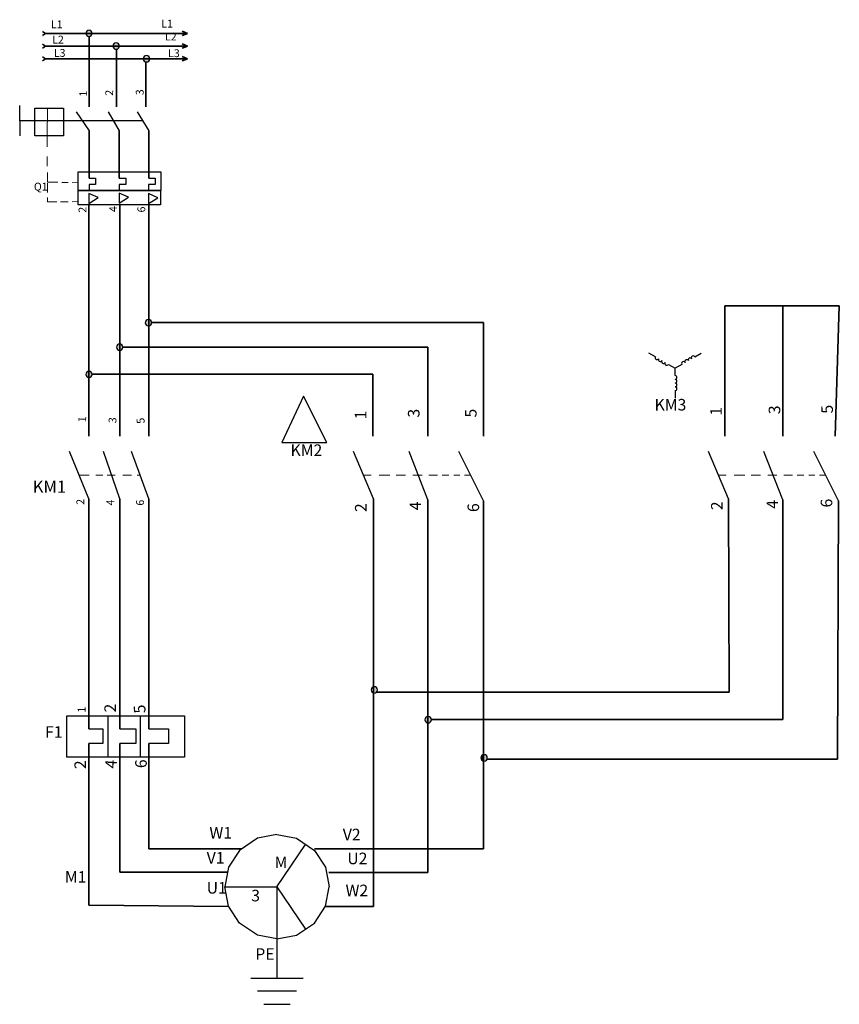
# Model space of a CAD drawing. Units: inches. Extents: x 4655 to 5300, y 4224 to 4998.
import ezdxf

# ---------------------------------------------------------------- set-up
doc = ezdxf.new("R2010")
doc.units = ezdxf.units.IN
doc.header["$MEASUREMENT"] = 0
for name, color, linetype, lineweight in [('E-ANNO-TEXT', 2, 'Continuous', 18), ('E-POWR-DEVC', 4, 'Continuous', 25), ('E-POWR-EQPM', 3, 'Continuous', 25), ('E-POWR-JUNC', 7, 'Continuous', 25), ('E-POWR-LINK', 8, 'Continuous', 18), ('E-POWR-WIRE', 7, 'Continuous', 35)]:
    doc.layers.add(name, color=color, linetype=linetype, lineweight=lineweight)
doc.styles.get("Standard").update_dxf_attribs({"font": 'arial.ttf'})

# ---------------------------------------------------------------- blocks, each defined once
blk = doc.blocks.new('Motor - 3-Phase WYE Grounded')
for p, q in [((-0.074922, 0.185436), (0, 0.199999)), ((0.074921, 0.185436), (0, 0.199999)), ((-0.138932, 0.143868), (-0.074922, 0.185436)), ((0.138931, 0.143868), (0.074921, 0.185436)), ((-0.185437, 0.074921), (-0.138932, 0.143868)), ((0.185436, 0.074921), (0.138931, 0.143868)), ((0, 0), (-0.162185, 0.109394)), ((0, 0), (0.162184, 0.109394)), ((0.349999, -0.1), (0.349999, 0.1)), ((-0.2, 0), (-0.185437, 0.074921)), ((0.199999, 0), (0.185436, 0.074921)), ((0.4, 0.075), (0.4, -0.075)), ((0.449999, -0.05), (0.449999, 0.05)), ((0, -0.2), (0, 0)), ((0, 0), (0.349999, 0)), ((-0.2, -0.000001), (-0.185437, -0.074922)), ((0.199999, -0.000001), (0.185436, -0.074922)), ((-0.185437, -0.074922), (-0.138932, -0.143869)), ((0.185436, -0.074922), (0.138931, -0.143869)), ((-0.138932, -0.143869), (-0.074922, -0.185437)), ((0.138931, -0.143869), (0.074921, -0.185437)), ((-0.074922, -0.185437), (0, -0.2)), ((0.074921, -0.185437), (0, -0.2))]:
    blk.add_line(p, q)
blk = doc.blocks.new('Transformer - WYE')
for p, q in [((-0.526796, 0.299999), (-0.700001, 0.4)), ((0.526795, 0.299999), (0.699999, 0.4)), ((-0.180385, 0.099999), (0, 0)), ((0.180384, 0.099999), (0, 0)), ((0, -0.2), (0, -0.000001)), ((0, -0.600001), (0, -0.800001))]:
    blk.add_line(p, q)
for centre, start, end in [((-0.483494, 0.275), 150, 330), ((0.396891, 0.224999), 29.99999, 210), ((0.483493, 0.274999), 29.99999, 210), ((-0.396892, 0.224999), 150, 330), ((-0.310289, 0.175), 150, 330), ((-0.223687, 0.125), 150, 330), ((0.223686, 0.125), 29.99999, 210), ((0.310288, 0.174999), 29.99999, 210), ((0, -0.25), 270, 90), ((0, -0.35), 270, 90), ((0, -0.45), 270, 90), ((0, -0.55), 270, 90)]:
    blk.add_arc(centre, 0.05, start, end)

msp = doc.modelspace()

# ---------------------------------------------------------------- hatches: boundary and pattern name
at = {"layer": 'E-POWR-JUNC'}
h = msp.add_hatch(color=256, dxfattribs=at)
h.dxf.hatch_style = 1
h.paths.add_polyline_path([(4757.35, 4967.74), (4752.35, 4967.74, 1)])
h.paths.add_polyline_path([(4752.35, 4967.74), (4757.35, 4967.74, 1)])
h.paths.add_polyline_path([(4733.51, 4977.74), (4728.51, 4977.74, 1)])
h.paths.add_polyline_path([(4728.51, 4977.74), (4733.51, 4977.74, 1)])
h.paths.add_polyline_path([(4712.12, 4987.74), (4707.12, 4987.74, 1)])
h.paths.add_polyline_path([(4707.12, 4987.74), (4712.12, 4987.74, 1)])
h = msp.add_hatch(color=256, dxfattribs=at)
h.dxf.hatch_style = 1
h.paths.add_polyline_path([(4756.55, 4762.71, 0.436019), (4753.86, 4760.21, 0.436019), (4756.55, 4757.72)])
h.paths.add_polyline_path([(4756.55, 4762.71), (4756.55, 4757.72, 0.392739), (4758.86, 4760.21, 0.392739)])
h.paths.add_polyline_path([(4733.82, 4743.51), (4733.82, 4738.51, 0.407781), (4736.26, 4741.01, 0.407781)])
h.paths.add_polyline_path([(4733.82, 4743.51, 0.420675), (4731.26, 4741.01, 0.420675), (4733.82, 4738.51)])
h.paths.add_polyline_path([(4709.55, 4722.08, 0.411018), (4707.08, 4719.58, 0.411018), (4709.55, 4717.08)])
h.paths.add_polyline_path([(4709.55, 4722.08), (4709.55, 4717.08, 0.417416), (4712.08, 4719.58, 0.417416)])
h = msp.add_hatch(color=256, dxfattribs=at)
h.dxf.hatch_style = 1
h.paths.add_polyline_path([(4933.51, 4473.96), (4933.51, 4469.07, 0.476905), (4936.53, 4471.52, 0.476905)])
h.paths.add_polyline_path([(4933.51, 4473.96, 0.354184), (4931.53, 4471.52, 0.354184), (4933.51, 4469.07)])
h.paths.add_polyline_path([(4976.22, 4450.52, 0.393918), (4973.89, 4448.03, 0.393918), (4976.22, 4445.53)])
h.paths.add_polyline_path([(4978.89, 4448.03, 0.434804), (4976.22, 4450.52), (4976.22, 4445.53, 0.434804)])
h.paths.add_polyline_path([(5019.94, 4420.5), (5019.94, 4415.58, 0.466925), (5022.88, 4418.04, 0.466925)])
h = msp.add_hatch(color=256, dxfattribs=at)
h.dxf.hatch_style = 1
h.paths.add_polyline_path([(5019.94, 4420.5, 0.363396), (5017.88, 4418.04, 0.363396), (5019.94, 4415.58)])

# ---------------------------------------------------------------- linework, layer by layer
at = {"layer": 'E-POWR-DEVC'}
for p, q in [((4655.08, 4919.01), (4655.08, 4931.09)), ((4699.59, 4925.99), (4709.69, 4911.08)), ((4724.71, 4925.99), (4733.41, 4911.08)), ((4747.58, 4925.99), (4756.54, 4911.08)), ((4751.77, 4919.01), (4655.08, 4919.01)), ((4655.08, 4919.01), (4655.08, 4907.17)), ((4709.69, 4873.81), (4714.79, 4873.81)), ((4714.79, 4873.81), (4714.79, 4868.91)), ((4733.41, 4873.81), (4738.45, 4873.81)), ((4738.45, 4873.81), (4738.45, 4868.91)), ((4756.54, 4873.81), (4761.61, 4873.81)), ((4761.61, 4873.81), (4761.61, 4868.91)), ((4709.69, 4868.91), (4709.66, 4864.1)), ((4714.79, 4868.91), (4709.69, 4868.91)), ((4733.34, 4868.91), (4733.32, 4864.1)), ((4738.45, 4868.91), (4733.34, 4868.91)), ((4733.43, 4862.18), (4733.43, 4854.15)), ((4740.6, 4858.82), (4733.43, 4862.18)), ((4756.5, 4868.91), (4756.48, 4864.1)), ((4761.61, 4868.91), (4756.5, 4868.91)), ((4709.54, 4861.93), (4709.54, 4853.9)), ((4716.71, 4858.56), (4709.54, 4861.93)), ((4709.54, 4853.9), (4716.71, 4858.56)), ((4733.43, 4854.15), (4740.6, 4858.82)), ((4756.49, 4861.86), (4756.49, 4853.84)), ((4763.66, 4858.5), (4756.49, 4861.86)), ((4756.49, 4853.84), (4763.66, 4858.5)), ((4709.55, 4621.66), (4694.31, 4658.96)), ((4733.82, 4621.66), (4720.93, 4658.96)), ((4756.55, 4621.66), (4743.12, 4658.96)), ((4933.51, 4621.66), (4917.69, 4658.96)), ((4976.22, 4620.9), (4961.33, 4658.96)), ((5019.94, 4620.12), (5000.53, 4658.96)), ((5212.73, 4621.66), (5196.9, 4658.96)), ((5255.43, 4620.9), (5240.54, 4658.96)), ((5299.15, 4620.12), (5279.74, 4658.96)), ((4724.33, 4451.08), (4724.33, 4418.61)), ((4749.98, 4451.08), (4749.98, 4418.61)), ((4709.55, 4440.86), (4720.4, 4440.86)), ((4720.4, 4440.86), (4720.4, 4429.35)), ((4733.82, 4440.86), (4746.37, 4440.86)), ((4746.37, 4440.86), (4746.37, 4429.35)), ((4756.55, 4440.86), (4772.05, 4440.86)), ((4772.05, 4440.86), (4772.05, 4429.35)), ((4720.4, 4429.35), (4709.55, 4429.35)), ((4746.37, 4429.35), (4733.82, 4429.35)), ((4772.05, 4429.35), (4756.55, 4429.35))]:
    msp.add_line(p, q, dxfattribs=at)
for points in [[(4666.95, 4928.97), (4689.54, 4928.97), (4689.54, 4907.14), (4666.95, 4907.14)], [(4700.95, 4878.73), (4765.98, 4878.73), (4765.98, 4864.1), (4700.95, 4864.1)], [(4700.95, 4864.1), (4765.94, 4864.1), (4765.94, 4852.93), (4700.95, 4852.93)], [(4692.23, 4451.08), (4784.77, 4451.08), (4784.77, 4418.61), (4692.23, 4418.61)]]:
    msp.add_lwpolyline(points, close=True, dxfattribs=at)
at = {"layer": 'E-POWR-EQPM'}
for p, q in [((4878.28, 4702.51), (4861.24, 4665.95)), ((4896.58, 4665.95), (4878.28, 4702.51)), ((4861.24, 4665.95), (4896.58, 4665.95))]:
    msp.add_line(p, q, dxfattribs=at)
at = {"layer": 'E-POWR-JUNC'}
for points in [[(4707.12, 4987.74, 1), (4712.12, 4987.74, 1)], [(4728.51, 4977.74, 1), (4733.51, 4977.74, 1)], [(4752.35, 4967.74, 1), (4757.35, 4967.74, 1)], [(4753.86, 4760.21, 1), (4758.86, 4760.21, 1)], [(4731.26, 4741.01, 1), (4736.26, 4741.01, 1)], [(4707.08, 4719.58, 1), (4712.08, 4719.58, 1)], [(4931.53, 4471.52, 1), (4936.53, 4471.52, 1)], [(4973.89, 4448.03, 1), (4978.89, 4448.03, 1)], [(5017.88, 4418.04, 1), (5022.88, 4418.04, 1)]]:
    msp.add_lwpolyline(points, format="xyb", close=True, dxfattribs=at)
at = {"layer": 'E-POWR-LINK'}
for p, q in [((4676.96, 4928.97), (4676.71, 4907.14)), ((4676.71, 4907.14), (4676.71, 4898.41)), ((4676.71, 4890.9), (4676.71, 4883.24)), ((4677, 4878.34), (4677, 4871.14)), ((4677, 4871.14), (4677, 4870.65)), ((4677, 4870.65), (4678.52, 4870.65)), ((4677.03, 4869.85), (4677.03, 4865.2)), ((4678.52, 4870.65), (4685.2, 4870.65)), ((4688.15, 4870.58), (4693.18, 4870.58)), ((4696.49, 4870.4), (4700.95, 4870.28)), ((4677.03, 4865.2), (4677.03, 4862.56)), ((4677.03, 4858.68), (4677.03, 4855.16)), ((4677.03, 4855.16), (4684.35, 4855.16)), ((4687.24, 4855.16), (4693.22, 4855.16)), ((4696.37, 4855.35), (4700.95, 4855.47)), ((4701.91, 4640.36), (4709.62, 4640.36)), ((4714.88, 4640.36), (4720.51, 4640.36)), ((4723.97, 4640.36), (4730.14, 4640.36)), ((4736.33, 4640.36), (4742.92, 4640.36)), ((4747.47, 4640.36), (4749.82, 4640.36)), ((4925.58, 4640.36), (4931.62, 4640.36)), ((4937.74, 4640.36), (4946.31, 4640.36)), ((4951.11, 4640.36), (4958.55, 4640.36)), ((4964.29, 4640.36), (4971.54, 4640.36)), ((4976.81, 4640.36), (4983.69, 4640.36)), ((4987.4, 4640.36), (4992.73, 4640.36)), ((4996.47, 4640.36), (5001.31, 4640.36)), ((5004.92, 4640.36), (5009.83, 4640.34)), ((5204.79, 4640.36), (5210.84, 4640.36)), ((5216.95, 4640.36), (5225.52, 4640.36)), ((5230.32, 4640.36), (5237.76, 4640.36)), ((5243.51, 4640.36), (5250.75, 4640.36)), ((5256.03, 4640.36), (5262.9, 4640.36)), ((5266.61, 4640.36), (5271.95, 4640.36)), ((5275.68, 4640.36), (5280.53, 4640.36)), ((5284.13, 4640.36), (5289.05, 4640.34))]:
    msp.add_line(p, q, dxfattribs=at)
at = {"layer": 'E-POWR-WIRE'}
for p, q in [((4675.3, 4987.74), (4673.03, 4989.17)), ((4675.3, 4987.74), (4673.03, 4986.03)), ((4675.3, 4987.74), (4787.06, 4987.74)), ((4787.06, 4987.74), (4782.76, 4989.54)), ((4787.06, 4987.74), (4782.76, 4986.04)), ((4675.3, 4977.74), (4673.03, 4979.17)), ((4709.69, 4985.24), (4709.69, 4929.86)), ((4787.06, 4977.74), (4782.76, 4979.54)), ((4675.3, 4977.74), (4673.03, 4976.03)), ((4675.3, 4977.74), (4787.06, 4977.74)), ((4731.15, 4975.24), (4731.15, 4929.86)), ((4787.06, 4977.74), (4782.76, 4976.04)), ((4675.3, 4967.74), (4673.03, 4969.17)), ((4675.3, 4967.74), (4673.03, 4966.03)), ((4675.3, 4967.74), (4787.06, 4967.74)), ((4754.35, 4965.29), (4754.35, 4929.86)), ((4787.06, 4967.74), (4782.76, 4969.54)), ((4787.06, 4967.74), (4782.76, 4966.04)), ((4709.69, 4911.08), (4709.69, 4873.81)), ((4733.41, 4911.08), (4733.41, 4873.81)), ((4756.54, 4911.08), (4756.54, 4873.81)), ((4709.55, 4852.93), (4709.55, 4670.93)), ((4733.82, 4852.93), (4733.82, 4670.93)), ((4756.55, 4852.93), (4756.55, 4670.93)), ((5209.64, 4671.02), (5209.64, 4773.62)), ((5209.64, 4773.62), (5299.79, 4773.62)), ((5255.48, 4671.02), (5255.24, 4773.62)), ((5299.79, 4773.62), (5296.63, 4671.02)), ((4758.86, 4760.3), (5019.94, 4760.3)), ((5019.94, 4760.3), (5019.94, 4671.02)), ((4736.26, 4741.1), (4976.1, 4741.1)), ((4976.1, 4741.1), (4976.1, 4671.02)), ((4712.08, 4719.67), (4932.84, 4719.67)), ((4932.84, 4719.67), (4932.84, 4671.02)), ((4709.55, 4621.66), (4709.55, 4440.86)), ((4733.82, 4621.66), (4733.82, 4440.86)), ((4756.55, 4621.66), (4756.55, 4440.86)), ((4933.51, 4301.19), (4933.51, 4621.66)), ((4976.22, 4620.9), (4976.22, 4328.05)), ((5019.94, 4346.64), (5019.94, 4620.12)), ((5212.73, 4621.66), (5213.06, 4469.64)), ((5255.43, 4620.9), (5255.41, 4448.13)), ((5299.15, 4620.12), (5298.31, 4416.96)), ((4935.66, 4469.62), (5213.06, 4469.64)), ((4978.89, 4448.13), (5255.41, 4448.13)), ((4709.55, 4429.35), (4709.55, 4302.25)), ((4733.82, 4429.35), (4733.82, 4328.21)), ((4756.55, 4429.35), (4756.55, 4346.64)), ((5022.63, 4416.96), (5298.31, 4416.96)), ((4756.55, 4346.64), (4829.9, 4346.64)), ((4887.02, 4346.64), (5019.94, 4346.64)), ((4733.82, 4328.21), (4818.58, 4328.13)), ((4898.2, 4328.05), (4976.22, 4328.05)), ((4709.55, 4302.25), (4819.45, 4301.19)), ((4895.46, 4301.19), (4933.51, 4301.19))]:
    msp.add_line(p, q, dxfattribs=at)

# ---------------------------------------------------------------- block references
at = {"layer": 'E-POWR-EQPM', "xscale": 29.44533644500327, "yscale": 29.44533644500327, "zscale": 29.44533644500327}
msp.add_blockref('Transformer - WYE', (5170.62, 4724.53), dxfattribs=at)
at = {"layer": 'E-POWR-EQPM', "xscale": 205.4678418545126, "yscale": 205.4678418545126, "zscale": 205.4678418545126, "rotation": 270}
msp.add_blockref('Motor - 3-Phase WYE Grounded', (4857.46, 4316.74), dxfattribs=at)

# ---------------------------------------------------------------- texts
at = {"layer": 'E-ANNO-TEXT'}
for s, height, p in [('L1', 6.152, (4679.59, 4991.74)), ('L1', 6.152, (4766.48, 4992.34)), ('L2', 6.152, (4680.59, 4979.76)), ('L2', 6.152, (4769.31, 4982.19)), ('L3', 6.152, (4681.92, 4969.27)), ('L3', 6.152, (4771.8, 4969.06)), ('Q1', 6.152, (4666.23, 4864.15)), ('KM3', 9.104, (5154.44, 4691.19)), ('KM2', 9.104, (4868.1, 4655.41)), ('KM1', 9.55, (4665.37, 4626.49)), ('F1', 9.104, (4675.07, 4433.86)), ('W1', 9.104, (4804.32, 4354.54)), ('V2', 9.104, (4909.22, 4353.2)), ('V1', 9.104, (4802.17, 4334.94)), ('U2', 9.104, (4912.77, 4334.42)), ('M', 9.1, (4855.6, 4331.37)), ('M1', 9.104, (4690.64, 4319.9)), ('U1', 9.104, (4802.17, 4311.3)), ('3', 9.1, (4837.2, 4305.23)), ('W2', 9.104, (4911.41, 4309.25)), ('PE', 9.104, (4840.4, 4259.25))]:
    msp.add_text(s, height=height, dxfattribs=at).set_placement(p)
for s, height, rotation, p in [('1', 6.15, 90.16465, (4708.16, 4938.08)), ('2', 6.15, 87.97022, (4728.49, 4938.55)), ('3', 6.15, 89.97783, (4752.59, 4939.12)), ('2', 6.15, 88.72598, (4707.47, 4846.59)), ('4', 6.15, 90.61016, (4731.69, 4847.24)), ('6', 6.15, 89.62966, (4753.81, 4846.88)), ('3', 9.1, 90, (4969.59, 4685.64)), ('5', 9.1, 90, (5014.46, 4685.64)), ('1', 9.1, 90.49957, (5207.37, 4687.2)), ('3', 9.1, 89.42344, (5253.29, 4688.25)), ('5', 9.1, 92.62185, (5294.89, 4688.96)), ('1', 6.15, 87.83452, (4707.25, 4681.83)), ('3', 6.15, 85.26256, (4730.97, 4680.97)), ('5', 6.15, 95.99163, (4753.5, 4681.14)), ('1', 9.1, 90, (4927.8, 4684.25)), ('2', 6.15, 90, (4705.85, 4617.04)), ('4', 6.15, 90, (4729.45, 4616.54)), ('6', 6.15, 90, (4752.83, 4616.39)), ('2', 9.1, 90, (4927.93, 4611.33)), ('4', 9.1, 90, (4970.85, 4612.72)), ('6', 9.1, 90, (5016.44, 4611.33)), ('2', 9.1, 90, (5207.99, 4612.83)), ('4', 9.1, 91.54848, (5251.77, 4614.04)), ('6', 9.1, 91.06283, (5294.32, 4615.01)), ('2', 9.1, 90.10204, (4730.8, 4453.75)), ('5', 9.1, 94.62152, (4754.23, 4453.35)), ('1', 6.15, 91.22497, (4706.96, 4453.69)), ('2', 9.1, 90.63595, (4707.29, 4409.28)), ('4', 9.1, 86.47887, (4731.2, 4409.5)), ('6', 9.1, 89.54434, (4755.01, 4409.94))]:
    msp.add_text(s, height=height, rotation=rotation, dxfattribs=at).set_placement(p)

doc.saveas('drawing.dxf')
